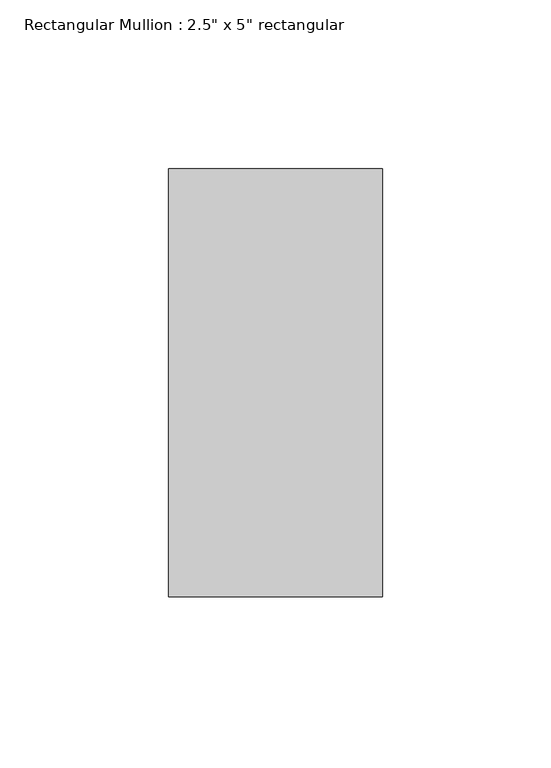
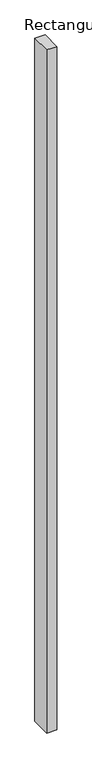
"""IFC4 building model written with IfcOpenShell, lengths in millimetres: member geometry."""

from ifc_helpers import new_model, si_unit, frame, origin, place, context, project, spatial, polyline, outline, extrude, source, transform, mapped, element, save


def member_ea77439e(model_context):
    return source(origin(), model_context, "Body", "SweptSolid", [
        extrude(outline(polyline([(0.0, 63.5), (0.0, -63.5), (-63.5, -63.5), (-63.5, 63.5), (0.0, 63.5)])), frame((0.0, 0.0, -4521.2), z_axis=(0.0, 0.0, 1.0), x_axis=(1.0, 0.0, 0.0)), (0.0, 0.0, 1.0), 4521.2),
    ])


if __name__ == "__main__":
    model = new_model("IFC4")
    model_context = context("Model", 3, world=origin())
    ifc_project = project(units=[si_unit("LENGTHUNIT", "METRE", prefix="MILLI")], contexts=[model_context])
    site = spatial("IfcSite", under=ifc_project)
    building = spatial("IfcBuilding", under=site)
    placement = place(None, origin())
    member_shape = member_ea77439e(model_context)
    element("IfcMember", 1, ObjectType="Rectangular Mullion : 2.5\" x 5\" rectangular", at=placement, inside=building, context=model_context, shape_type="MappedRepresentation", body=[
        mapped(member_shape, transform((0.0, 0.0, 0.0), x_axis=(1.0, 0.0, 0.0), y_axis=(0.0, 1.0, 0.0), z_axis=(0.0, 0.0, 1.0))),
    ])
    save(model, "model.ifc")

# Revit data of these elements
# Type "Rectangular Mullion : 2.5\" x 5\" rectangular"
#   built-in parameter 1007304 = 0.416667 (stored number, unit not read)
#   built-in parameter 1007301 = 0.104167 (stored number, unit not read)
#   built-in parameter 1007300 = 0.104167 (stored number, unit not read)
# Element 1 (IfcMember, "Rectangular Mullion : 2.5\" x 5\" rectangular")
#   Materials on its faces: "Aluminum"
# Materials
#   "Aluminum": class "Metal", colour RGB 247 247 247, transparency 0, Description = "Aluminum 6061", Cost = 0
